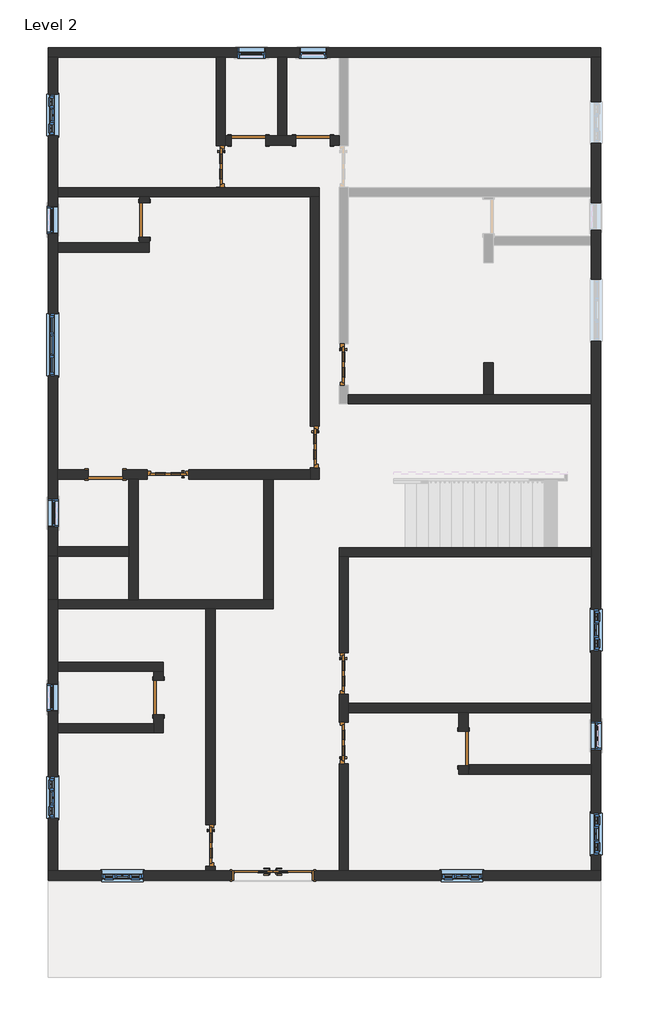
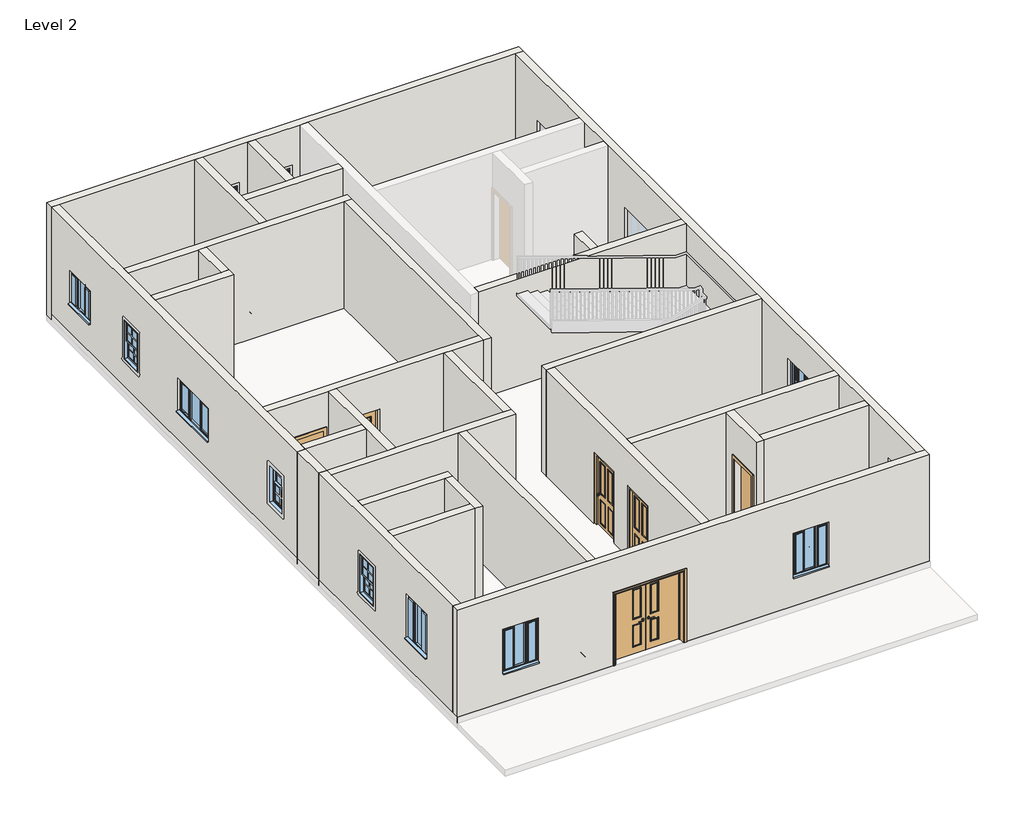
# One storey, part 1 of 3: 29 walls, 14 doors, 13 windows.
# Revit data of these elements (continued)
# Type "Windows_Tpl_w-Glazing_Cross-Bars : 910x1210mm"
#   Type Mark = "25"
#   Operation = "TriplePanelVertical"
#   Construction Type Id = "GSP4R"
#   Manufacturer = "Revit"
#   Keynote = "L10"
#   Analytic Construction = "1/8 in Pilkington single glazing"
#   Wrap Layers (Ext) from Ext = 0' - 4.03543"
#   Wrap Layers (Int) from Ext = 0' - 6.98819"
#   Window Board Projection = 0' - 0.98425"
#   Window Board Extension = 0' - 0.98425"
#   Visual Light Transmittance = 0.9
#   Solar Heat Gain Coefficient = 0.78
#   Rough Width = 2' - 11.82677"
#   Rough Height = 3' - 11.6378"
#   Height = 3' - 11.6378"
#   Width = 2' - 11.82677"
#   Heat Transfer Coefficient (U) = 0.6496 BTU/(h·ft²·°F)
#   Glazing Thickness = 0' - 0.94488"
#   Glazing Bar Thickness = 0' - 0.7874"
#   FrameOffset - External = 0' - 1.9685"
#   Frame Depth = 0' - 2.55906"
#   Default Head Height = 6' - 11.07087"
#   Cill Depth = 0' - 3.44488"
#   Cavity Closer Width = 0' - 1.9685"
#   Cavity Closer Offset from Ext = 0' - 4.03543"
#   Cavity Closer Depth = 0' - 3.34646"
#   Vis - Glazing Bars = yes
#   Vis - Cavity Closers = yes
#   Define Thermal Properties by = 1
#   Material Trim = Window Frame
#   Material Glazing Bars = Window Frame
#   Material Glass = Glass
#   Material Frame = Window Frame
#   Wall Closure = (empty or 0)
# Type "Windows_Tpl_w-Glazing_Cross-Bars : 910x910mm"
#   Type Mark = "24"
#   Operation = "TriplePanelVertical"
#   Construction Type Id = "GSP4R"
#   Manufacturer = "Revit"
#   Keynote = "L10"
#   Analytic Construction = "1/8 in Pilkington single glazing"
#   Wrap Layers (Ext) from Ext = 0' - 4.03543"
#   Wrap Layers (Int) from Ext = 0' - 6.98819"
#   Window Board Projection = 0' - 0.98425"
#   Window Board Extension = 0' - 0.98425"
#   Visual Light Transmittance = 0.9
#   Solar Heat Gain Coefficient = 0.78
#   Rough Width = 2' - 11.82677"
#   Rough Height = 2' - 11.82677"
#   Height = 2' - 11.82677"
#   Width = 2' - 11.82677"
#   Heat Transfer Coefficient (U) = 0.6496 BTU/(h·ft²·°F)
#   Glazing Thickness = 0' - 0.94488"
#   Glazing Bar Thickness = 0' - 0.7874"
#   FrameOffset - External = 0' - 1.9685"
#   Frame Depth = 0' - 2.55906"
#   Default Head Height = 6' - 11.07087"
#   Cill Depth = 0' - 3.44488"
#   Cavity Closer Width = 0' - 1.9685"
#   Cavity Closer Offset from Ext = 0' - 4.03543"
#   Cavity Closer Depth = 0' - 3.34646"
#   Vis - Glazing Bars = yes
#   Vis - Cavity Closers = yes
#   Define Thermal Properties by = 1
#   Material Trim = Window Frame
#   Material Glazing Bars = Window Frame
#   Material Glass = Glass
#   Material Frame = Window Frame
#   Wall Closure = (empty or 0)
# Elements 1, 2, 3, 4, 5, 6, 7 (IfcDoor, "Doors_ExtSgl_2 : 2'x7\"")
#   Phase Created = New Construction
#   Materials on its faces: "Door - Panel", "Door - Handle", "Door - Frame/Mullion", "Door - Glazing"
# Element 8 (IfcDoor, "Doors_IntDbl_3 : 1810x2110mm")
#   Phase Created = New Construction
#   Materials on its faces: "Door - Panel", "Door - Handle", "Door - Architrave", "Door - Frame/Mullion", "Door - Glazing"
# Elements 9, 10, 11, 12, 13, 14 (IfcDoor, "Single-Flush : 30\" x 80\"")
#   Phase Created = New Construction
#   Materials on its faces: "Door - Frame", "Door - Panel"
# Elements 15, 16, 17, 18, 19, 20, 21, 22, 23, 24, 25, 26, 27, 28, 29, 30, 31, 32, 33, 34, 35, 36, 37 (IfcWall, "Generic - 4.5\" p")
#   Top Offset = 0' - 0"
#   Base Offset = 0' - 0"
#   Unconnected Height = 10' - 0"
#   wall height = 10' - 0"
#   Phase Created = New Construction
#   Base Constraint = Level 2
#   Materials on its faces: "Default Wall"
# Element 38 (IfcWall, "Generic - 4.5\" p")
#   Top Offset = 0' - 0"
#   Base Offset = 0' - 0"
#   Unconnected Height = 10' - 0"
#   wall height = 10' - 0"
#   Phase Created = New Construction
#   Base Constraint = Level 2
#   Materials on its faces: "Default Wall", "Door - Panel"
# Elements 39, 41, 42, 43 (IfcWall, "Generic - 9\" w")
#   Top Offset = 0' - 0"
#   Base Offset = 0' - 0"
#   Unconnected Height = 10' - 0"
#   wall height = 10' - 0"
#   Phase Created = New Construction
#   Base Constraint = Level 2
#   Materials on its faces: "Default Wall", "Door - Panel"
# Element 40 (IfcWall, "Generic - 9\" w")
#   Top Offset = 0' - 0"
#   Base Offset = 0' - 0"
#   Unconnected Height = 10' - 0"
#   wall height = 10' - 0"
#   Phase Created = New Construction
#   Base Constraint = Level 2
#   Materials on its faces: "Default Wall", "Door - Panel", "Default Mass Interior Wall"
# Element 44 (IfcWindow, "Window-Double-Hung : 24\" x 42\"")
#   Mark = "10"
#   Window Inset = 0' - 0"
#   Interior Wall Closure = 0' - 1 1/2"
#   Frame Extension = 0' - 1 1/4"
#   Exterior Wall Closure = 0' - 0 1/2"
#   Interior Trim Visibility = yes
#   Indicator Visibility = yes
#   Exterior Trim Visibility = yes
#   Phase Created = New Construction
#   Materials on its faces: "Wood - Stained", "Glass", "Clad - White"
# Element 45 (IfcWindow, "Window-Double-Hung : 24\" x 42\"")
#   Mark = "11"
#   Window Inset = 0' - 0"
#   Interior Wall Closure = 0' - 1 1/2"
#   Frame Extension = 0' - 1 1/4"
#   Exterior Wall Closure = 0' - 0 1/2"
#   Interior Trim Visibility = yes
#   Indicator Visibility = yes
#   Exterior Trim Visibility = yes
#   Phase Created = New Construction
#   Materials on its faces: "Wood - Stained", "Glass", "Clad - White"
# Element 46 (IfcWindow, "Window-Double-Hung : 24\" x 42\"")
#   Mark = "12"
#   Window Inset = 0' - 0"
#   Interior Wall Closure = 0' - 1 1/2"
#   Frame Extension = 0' - 1 1/4"
#   Exterior Wall Closure = 0' - 0 1/2"
#   Interior Trim Visibility = yes
#   Indicator Visibility = yes
#   Exterior Trim Visibility = yes
#   Phase Created = New Construction
#   Materials on its faces: "Wood - Stained", "Glass", "Clad - White"
# Element 47 (IfcWindow, "Window-Double-Hung : 24\" x 42\"")
#   Mark = "14"
#   Window Inset = 0' - 0"
#   Interior Wall Closure = 0' - 1 1/2"
#   Frame Extension = 0' - 1 1/4"
#   Exterior Wall Closure = 0' - 0 1/2"
#   Interior Trim Visibility = yes
#   Indicator Visibility = yes
#   Exterior Trim Visibility = yes
#   Phase Created = New Construction
#   Materials on its faces: "Wood - Stained", "Glass", "Clad - White"
# Element 48 (IfcWindow, "Window-Double-Hung : 24\" x 42\"")
#   Mark = "15"
#   Window Inset = 0' - 0"
#   Interior Wall Closure = 0' - 1 1/2"
#   Frame Extension = 0' - 1 1/4"
#   Exterior Wall Closure = 0' - 0 1/2"
#   Interior Trim Visibility = yes
#   Indicator Visibility = yes
#   Exterior Trim Visibility = yes
#   Phase Created = New Construction
#   Materials on its faces: "Wood - Stained", "Glass", "Clad - White"
# Element 49 (IfcWindow, "Window-Double-Hung : 24\" x 42\"")
#   Mark = "16"
#   Window Inset = 0' - 0"
#   Interior Wall Closure = 0' - 1 1/2"
#   Frame Extension = 0' - 1 1/4"
#   Exterior Wall Closure = 0' - 0 1/2"
#   Interior Trim Visibility = yes
#   Indicator Visibility = yes
#   Exterior Trim Visibility = yes
#   Phase Created = New Construction
#   Materials on its faces: "Wood - Stained", "Glass", "Clad - White"
# Element 50 (IfcWindow, "Windows_Tpl_Plain : 1360x910mm")
#   Mark = "7"
#   Phase Created = New Construction
#   Materials on its faces: "Window Frame", "Glass"
# Element 51 (IfcWindow, "Windows_Tpl_w-Glazing_Cross-Bars : 910x1210mm")
#   Mark = "1"
#   Phase Created = New Construction
#   Materials on its faces: "Window Frame", "Glass"
# Element 52 (IfcWindow, "Windows_Tpl_w-Glazing_Cross-Bars : 910x1210mm")
#   Mark = "2"
#   Phase Created = New Construction
#   Materials on its faces: "Window Frame", "Glass"
# Element 53 (IfcWindow, "Windows_Tpl_w-Glazing_Cross-Bars : 910x1210mm")
#   Mark = "3"
#   Phase Created = New Construction
#   Materials on its faces: "Window Frame", "Glass"
# Element 54 (IfcWindow, "Windows_Tpl_w-Glazing_Cross-Bars : 910x1210mm")
#   Mark = "4"
#   Phase Created = New Construction
#   Materials on its faces: "Window Frame", "Glass"
# Element 55 (IfcWindow, "Windows_Tpl_w-Glazing_Cross-Bars : 910x1210mm")
#   Mark = "5"
#   Phase Created = New Construction
#   Materials on its faces: "Window Frame", "Glass"
# Element 56 (IfcWindow, "Windows_Tpl_w-Glazing_Cross-Bars : 910x910mm")
#   Mark = "8"
#   Phase Created = New Construction
#   Materials on its faces: "Window Frame", "Glass"
# Materials
#   "Door - Glazing": colour RGB 0 0 255, transparency 0.75
#   "Door - Panel": class "Wood", colour RGB 210 159 95, transparency 0, Cost = 0
#   "Door - Frame/Mullion": class "Wood", colour RGB 212 179 113, transparency 0
#   "Door - Handle": colour RGB 246 240 166, transparency 0
#   "Door - Architrave": class "Wood", colour RGB 154 90 5, transparency 0
#   "Door - Frame": colour RGB 118 70 51, transparency 0, Cost = 0
#   "Wood - Stained": class "Wood", colour RGB 224 178 126, transparency 0, Cost = 0
#   "Clad - White": class "Wood", colour RGB 242 242 238, transparency 0, Cost = 0
#   "Glass": class "Glass", colour RGB 0 128 192, transparency 0.75, Description = "Soda Lime Glass", Cost = 0
#   "Window Frame": colour RGB 249 249 249, transparency 0
#   "Default Wall": colour RGB 128 128 128, transparency 0, Cost = 0
#   "Default Mass Interior Wall": class "Generic", colour RGB 195 229 126, transparency 0, Cost = 0
